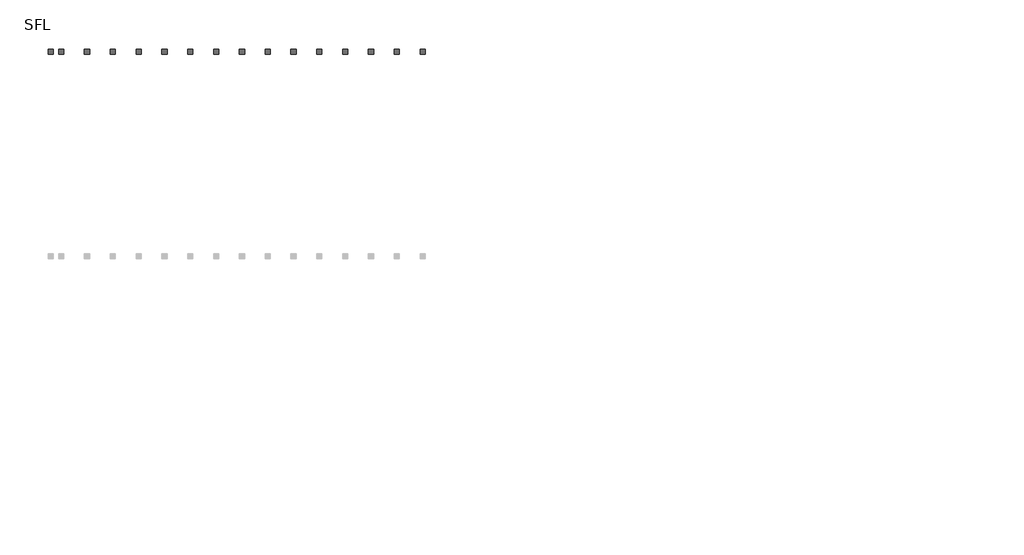
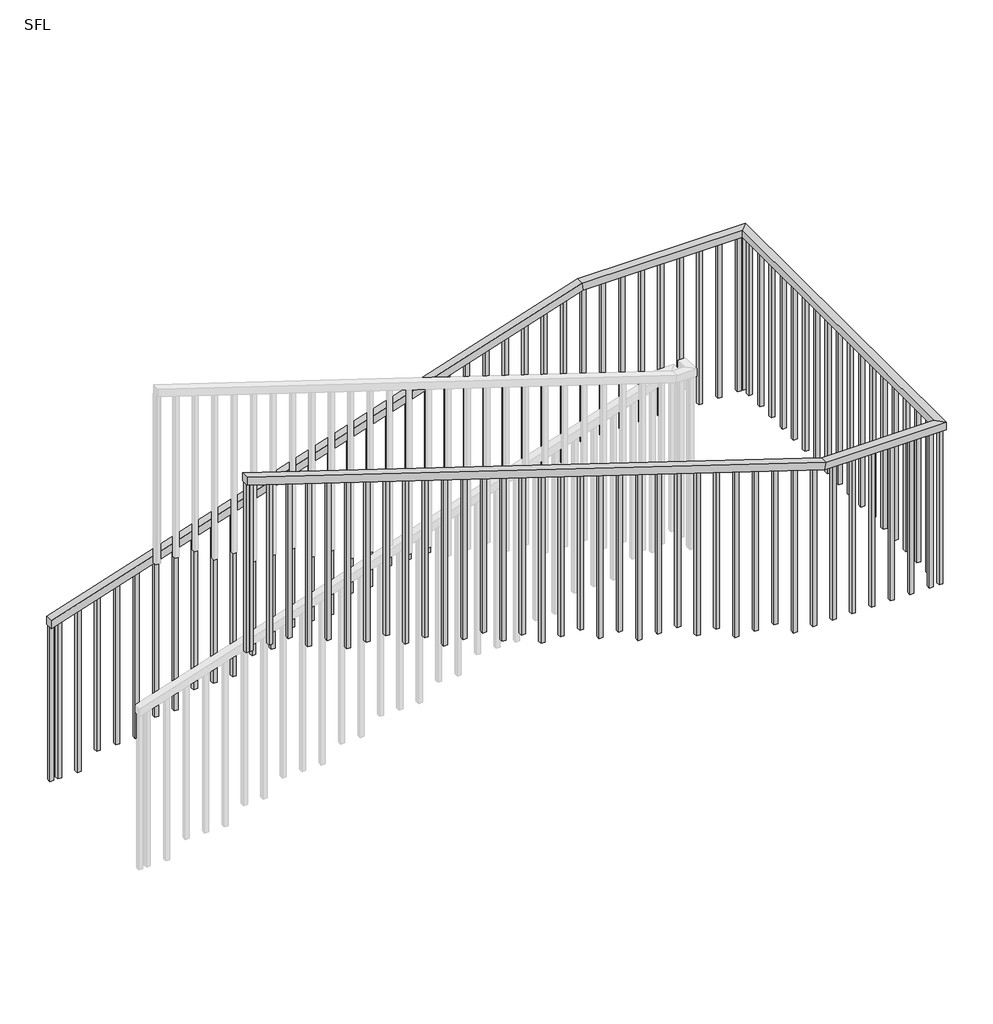
# One storey, part 2 of 2: 1 railing.
"""IFC4 building model written with IfcOpenShell, lengths in millimetres."""

from ifc_helpers import new_model, si_unit, frame, origin, place, context, project, spatial, polyline, outline, extrude, faceted_brep, element, save

model = new_model("IFC4")

# Units and contexts
model_context = context("Model", 3, world=origin())
ifc_project = project(units=[si_unit("LENGTHUNIT", "METRE", prefix="MILLI")], contexts=[model_context])

# Site, building, storey
site = spatial("IfcSite", under=ifc_project)
building = spatial("IfcBuilding", under=site)
storey = spatial("IfcBuildingStorey", under=building, Name="SFL", Elevation=6000.0)

# Railing
placement = place(None, origin())
element("IfcRailing", 1, ObjectType="1100mm", at=placement, inside=storey, context=model_context, shape_type="SolidModel", body=[
    faceted_brep([(-40149.9681829, 17835.7234223, 7799.9767904), (-40149.9681829, 17835.7234223, 7747.4487757), (-40149.9681829, 17785.7234223, 7747.4487757), (-40149.9681829, 17785.7234223, 7799.9767904), (-36733.6681829, 17835.7234223, 8899.9878906), (-36725.8169379, 17835.7234223, 8849.9878906), (-36725.8169379, 17785.7234223, 8849.9878906), (-36733.6681829, 17785.7234223, 8899.9878906), (-35651.74796, 17835.7234223, 8899.9878906), (-35651.74796, 17835.7234223, 8849.9878906), (-35701.74796, 17785.7234223, 8849.9878906), (-35701.74796, 17785.7234223, 8899.9878906), (-35651.74796, 15601.3234223, 8899.9878906), (-35651.74796, 15601.3234223, 8849.9878906), (-35701.74796, 15651.3234223, 8849.9878906), (-35701.74796, 15651.3234223, 8899.9878906), (-36423.0954556, 15601.3234223, 8899.9878906), (-36430.9467006, 15601.3234223, 8849.9878906), (-36430.9467006, 15651.3234223, 8849.9878906), (-36423.0954556, 15651.3234223, 8899.9878906), (-40149.9681829, 15601.3234223, 10100.0), (-40149.9681829, 15651.3234223, 10100.0), (-40149.9681829, 15651.3234223, 10047.4719853), (-40149.9681829, 15601.3234223, 10047.4719853)], [[[0, 1, 2, 3]], [[1, 0, 4, 5]], [[2, 1, 5, 6]], [[3, 2, 6, 7]], [[0, 3, 7, 4]], [[5, 4, 8, 9]], [[6, 5, 9, 10]], [[7, 6, 10, 11]], [[4, 7, 11, 8]], [[9, 8, 12, 13]], [[10, 9, 13, 14]], [[11, 10, 14, 15]], [[8, 11, 15, 12]], [[13, 12, 16, 17]], [[14, 13, 17, 18]], [[15, 14, 18, 19]], [[12, 15, 19, 16]], [[20, 21, 22, 23]], [[17, 16, 20, 23]], [[18, 17, 23, 22]], [[19, 18, 22, 21]], [[16, 19, 21, 20]]]),
    extrude(outline(polyline([(10031.9456028, -40101.74796), (10039.9953284, -40126.74796), (8899.9989909, -40126.74796), (8899.9989909, -40101.74796), (10031.9456028, -40101.74796)])), frame((0.0, 15613.8234223, 0.0), z_axis=(0.0, 1.0, 0.0), x_axis=(0.0, 0.0, 1.0)), (0.0, 0.0, 1.0), 25.0),
    extrude(outline(polyline([(9991.6969749, -39976.74796), (9999.7467005, -40001.74796), (8899.9989909, -40001.74796), (8899.9989909, -39976.74796), (9991.6969749, -39976.74796)])), frame((0.0, 15613.8234223, 0.0), z_axis=(0.0, 1.0, 0.0), x_axis=(0.0, 0.0, 1.0)), (0.0, 0.0, 1.0), 25.0),
    extrude(outline(polyline([(9951.448347, -39851.74796), (9959.4980726, -39876.74796), (8899.9989909, -39876.74796), (8899.9989909, -39851.74796), (9951.448347, -39851.74796)])), frame((0.0, 15613.8234223, 0.0), z_axis=(0.0, 1.0, 0.0), x_axis=(0.0, 0.0, 1.0)), (0.0, 0.0, 1.0), 25.0),
    extrude(outline(polyline([(9911.1997191, -39726.74796), (9919.2494447, -39751.74796), (8799.9979818, -39751.74796), (8799.9979818, -39726.74796), (9911.1997191, -39726.74796)])), frame((0.0, 15613.8234223, 0.0), z_axis=(0.0, 1.0, 0.0), x_axis=(0.0, 0.0, 1.0)), (0.0, 0.0, 1.0), 25.0),
    extrude(outline(polyline([(9870.9510912, -39601.74796), (9879.0008168, -39626.74796), (8799.9979818, -39626.74796), (8799.9979818, -39601.74796), (9870.9510912, -39601.74796)])), frame((0.0, 15613.8234223, 0.0), z_axis=(0.0, 1.0, 0.0), x_axis=(0.0, 0.0, 1.0)), (0.0, 0.0, 1.0), 25.0),
    extrude(outline(polyline([(9830.7024633, -39476.74796), (9838.7521889, -39501.74796), (8699.9969727, -39501.74796), (8699.9969727, -39476.74796), (9830.7024633, -39476.74796)])), frame((0.0, 15613.8234223, 0.0), z_axis=(0.0, 1.0, 0.0), x_axis=(0.0, 0.0, 1.0)), (0.0, 0.0, 1.0), 25.0),
    extrude(outline(polyline([(9790.4538354, -39351.74796), (9798.503561, -39376.74796), (8699.9969727, -39376.74796), (8699.9969727, -39351.74796), (9790.4538354, -39351.74796)])), frame((0.0, 15613.8234223, 0.0), z_axis=(0.0, 1.0, 0.0), x_axis=(0.0, 0.0, 1.0)), (0.0, 0.0, 1.0), 25.0),
    extrude(outline(polyline([(9750.2052075, -39226.74796), (9758.254933, -39251.74796), (8699.9969727, -39251.74796), (8699.9969727, -39226.74796), (9750.2052075, -39226.74796)])), frame((0.0, 15613.8234223, 0.0), z_axis=(0.0, 1.0, 0.0), x_axis=(0.0, 0.0, 1.0)), (0.0, 0.0, 1.0), 25.0),
    extrude(outline(polyline([(9710.0216346, -39101.74796), (9718.0713601, -39126.74796), (8599.9959635, -39126.74796), (8599.9959635, -39101.74796), (9710.0216346, -39101.74796)])), frame((0.0, 15613.8234223, 0.0), z_axis=(0.0, 1.0, 0.0), x_axis=(0.0, 0.0, 1.0)), (0.0, 0.0, 1.0), 25.0),
    extrude(outline(polyline([(9669.7730066, -38976.74796), (9677.8227322, -39001.74796), (8599.9959635, -39001.74796), (8599.9959635, -38976.74796), (9669.7730066, -38976.74796)])), frame((0.0, 15613.8234223, 0.0), z_axis=(0.0, 1.0, 0.0), x_axis=(0.0, 0.0, 1.0)), (0.0, 0.0, 1.0), 25.0),
    extrude(outline(polyline([(9629.5243787, -38851.74796), (9637.5741043, -38876.74796), (8499.9949544, -38876.74796), (8499.9949544, -38851.74796), (9629.5243787, -38851.74796)])), frame((0.0, 15613.8234223, 0.0), z_axis=(0.0, 1.0, 0.0), x_axis=(0.0, 0.0, 1.0)), (0.0, 0.0, 1.0), 25.0),
    extrude(outline(polyline([(9589.2757508, -38726.74796), (9597.3254764, -38751.74796), (8499.9949544, -38751.74796), (8499.9949544, -38726.74796), (9589.2757508, -38726.74796)])), frame((0.0, 15613.8234223, 0.0), z_axis=(0.0, 1.0, 0.0), x_axis=(0.0, 0.0, 1.0)), (0.0, 0.0, 1.0), 25.0),
    extrude(outline(polyline([(9549.0271229, -38601.74796), (9557.0768485, -38626.74796), (8499.9949544, -38626.74796), (8499.9949544, -38601.74796), (9549.0271229, -38601.74796)])), frame((0.0, 15613.8234223, 0.0), z_axis=(0.0, 1.0, 0.0), x_axis=(0.0, 0.0, 1.0)), (0.0, 0.0, 1.0), 25.0),
    extrude(outline(polyline([(9508.778495, -38476.74796), (9516.8282206, -38501.74796), (8399.9939453, -38501.74796), (8399.9939453, -38476.74796), (9508.778495, -38476.74796)])), frame((0.0, 15613.8234223, 0.0), z_axis=(0.0, 1.0, 0.0), x_axis=(0.0, 0.0, 1.0)), (0.0, 0.0, 1.0), 25.0),
    extrude(outline(polyline([(9468.5298671, -38351.74796), (9476.5795927, -38376.74796), (8399.9939453, -38376.74796), (8399.9939453, -38351.74796), (9468.5298671, -38351.74796)])), frame((0.0, 15613.8234223, 0.0), z_axis=(0.0, 1.0, 0.0), x_axis=(0.0, 0.0, 1.0)), (0.0, 0.0, 1.0), 25.0),
    extrude(outline(polyline([(9428.2812392, -38226.74796), (9436.3309648, -38251.74796), (8299.9929362, -38251.74796), (8299.9929362, -38226.74796), (9428.2812392, -38226.74796)])), frame((0.0, 15613.8234223, 0.0), z_axis=(0.0, 1.0, 0.0), x_axis=(0.0, 0.0, 1.0)), (0.0, 0.0, 1.0), 25.0),
    extrude(outline(polyline([(9388.0326113, -38101.74796), (9396.0823368, -38126.74796), (8299.9929362, -38126.74796), (8299.9929362, -38101.74796), (9388.0326113, -38101.74796)])), frame((0.0, 15613.8234223, 0.0), z_axis=(0.0, 1.0, 0.0), x_axis=(0.0, 0.0, 1.0)), (0.0, 0.0, 1.0), 25.0),
    extrude(outline(polyline([(9347.7839834, -37976.74796), (9355.8337089, -38001.74796), (8299.9929362, -38001.74796), (8299.9929362, -37976.74796), (9347.7839834, -37976.74796)])), frame((0.0, 15613.8234223, 0.0), z_axis=(0.0, 1.0, 0.0), x_axis=(0.0, 0.0, 1.0)), (0.0, 0.0, 1.0), 25.0),
    extrude(outline(polyline([(9307.5353554, -37851.74796), (9315.585081, -37876.74796), (8199.9919271, -37876.74796), (8199.9919271, -37851.74796), (9307.5353554, -37851.74796)])), frame((0.0, 15613.8234223, 0.0), z_axis=(0.0, 1.0, 0.0), x_axis=(0.0, 0.0, 1.0)), (0.0, 0.0, 1.0), 25.0),
    extrude(outline(polyline([(9267.2867275, -37726.74796), (9275.3364531, -37751.74796), (8199.9919271, -37751.74796), (8199.9919271, -37726.74796), (9267.2867275, -37726.74796)])), frame((0.0, 15613.8234223, 0.0), z_axis=(0.0, 1.0, 0.0), x_axis=(0.0, 0.0, 1.0)), (0.0, 0.0, 1.0), 25.0),
    extrude(outline(polyline([(9227.0380996, -37601.74796), (9235.0878252, -37626.74796), (8099.990918, -37626.74796), (8099.990918, -37601.74796), (9227.0380996, -37601.74796)])), frame((0.0, 15613.8234223, 0.0), z_axis=(0.0, 1.0, 0.0), x_axis=(0.0, 0.0, 1.0)), (0.0, 0.0, 1.0), 25.0),
    extrude(outline(polyline([(9186.7894717, -37476.74796), (9194.8391973, -37501.74796), (8099.990918, -37501.74796), (8099.990918, -37476.74796), (9186.7894717, -37476.74796)])), frame((0.0, 15613.8234223, 0.0), z_axis=(0.0, 1.0, 0.0), x_axis=(0.0, 0.0, 1.0)), (0.0, 0.0, 1.0), 25.0),
    extrude(outline(polyline([(9146.5408438, -37351.74796), (9154.5905694, -37376.74796), (8099.990918, -37376.74796), (8099.990918, -37351.74796), (9146.5408438, -37351.74796)])), frame((0.0, 15613.8234223, 0.0), z_axis=(0.0, 1.0, 0.0), x_axis=(0.0, 0.0, 1.0)), (0.0, 0.0, 1.0), 25.0),
    extrude(outline(polyline([(9106.2922159, -37226.74796), (9114.3419415, -37251.74796), (7999.9899089, -37251.74796), (7999.9899089, -37226.74796), (9106.2922159, -37226.74796)])), frame((0.0, 15613.8234223, 0.0), z_axis=(0.0, 1.0, 0.0), x_axis=(0.0, 0.0, 1.0)), (0.0, 0.0, 1.0), 25.0),
    extrude(outline(polyline([(9066.043588, -37101.74796), (9074.0933136, -37126.74796), (7999.9899089, -37126.74796), (7999.9899089, -37101.74796), (9066.043588, -37101.74796)])), frame((0.0, 15613.8234223, 0.0), z_axis=(0.0, 1.0, 0.0), x_axis=(0.0, 0.0, 1.0)), (0.0, 0.0, 1.0), 25.0),
    extrude(outline(polyline([(9025.7949601, -36976.74796), (9033.8446856, -37001.74796), (7899.9888997, -37001.74796), (7899.9888997, -36976.74796), (9025.7949601, -36976.74796)])), frame((0.0, 15613.8234223, 0.0), z_axis=(0.0, 1.0, 0.0), x_axis=(0.0, 0.0, 1.0)), (0.0, 0.0, 1.0), 25.0),
    extrude(outline(polyline([(8985.5463322, -36851.74796), (8993.5960577, -36876.74796), (7899.9888997, -36876.74796), (7899.9888997, -36851.74796), (8985.5463322, -36851.74796)])), frame((0.0, 15613.8234223, 0.0), z_axis=(0.0, 1.0, 0.0), x_axis=(0.0, 0.0, 1.0)), (0.0, 0.0, 1.0), 25.0),
    extrude(outline(polyline([(8945.2977042, -36726.74796), (8953.3474298, -36751.74796), (7899.9888997, -36751.74796), (7899.9888997, -36726.74796), (8945.2977042, -36726.74796)])), frame((0.0, 15613.8234223, 0.0), z_axis=(0.0, 1.0, 0.0), x_axis=(0.0, 0.0, 1.0)), (0.0, 0.0, 1.0), 25.0),
    extrude(outline(polyline([(8905.0490763, -36601.74796), (8913.0988019, -36626.74796), (7799.9878906, -36626.74796), (7799.9878906, -36601.74796), (8905.0490763, -36601.74796)])), frame((0.0, 15613.8234223, 0.0), z_axis=(0.0, 1.0, 0.0), x_axis=(0.0, 0.0, 1.0)), (0.0, 0.0, 1.0), 25.0),
    extrude(outline(polyline([(8864.8004484, -36476.74796), (8872.850174, -36501.74796), (7799.9878906, -36501.74796), (7799.9878906, -36476.74796), (8864.8004484, -36476.74796)])), frame((0.0, 15613.8234223, 0.0), z_axis=(0.0, 1.0, 0.0), x_axis=(0.0, 0.0, 1.0)), (0.0, 0.0, 1.0), 25.0),
    extrude(outline(polyline([(-36351.74796, 15613.8234223), (-36376.74796, 15613.8234223), (-36376.74796, 15638.8234223), (-36351.74796, 15638.8234223), (-36351.74796, 15613.8234223)])), frame((0.0, 0.0, 7799.9878906), z_axis=(0.0, 0.0, 1.0), x_axis=(1.0, 0.0, 0.0)), (0.0, 0.0, 1.0), 1050.0),
    extrude(outline(polyline([(-36226.74796, 15613.8234223), (-36251.74796, 15613.8234223), (-36251.74796, 15638.8234223), (-36226.74796, 15638.8234223), (-36226.74796, 15613.8234223)])), frame((0.0, 0.0, 7799.9878906), z_axis=(0.0, 0.0, 1.0), x_axis=(1.0, 0.0, 0.0)), (0.0, 0.0, 1.0), 1050.0),
    extrude(outline(polyline([(-36101.74796, 15613.8234223), (-36126.74796, 15613.8234223), (-36126.74796, 15638.8234223), (-36101.74796, 15638.8234223), (-36101.74796, 15613.8234223)])), frame((0.0, 0.0, 7799.9878906), z_axis=(0.0, 0.0, 1.0), x_axis=(1.0, 0.0, 0.0)), (0.0, 0.0, 1.0), 1050.0),
    extrude(outline(polyline([(-35976.74796, 15613.8234223), (-36001.74796, 15613.8234223), (-36001.74796, 15638.8234223), (-35976.74796, 15638.8234223), (-35976.74796, 15613.8234223)])), frame((0.0, 0.0, 7799.9878906), z_axis=(0.0, 0.0, 1.0), x_axis=(1.0, 0.0, 0.0)), (0.0, 0.0, 1.0), 1050.0),
    extrude(outline(polyline([(-35851.74796, 15613.8234223), (-35876.74796, 15613.8234223), (-35876.74796, 15638.8234223), (-35851.74796, 15638.8234223), (-35851.74796, 15613.8234223)])), frame((0.0, 0.0, 7799.9878906), z_axis=(0.0, 0.0, 1.0), x_axis=(1.0, 0.0, 0.0)), (0.0, 0.0, 1.0), 1050.0),
    extrude(outline(polyline([(-35726.74796, 15613.8234223), (-35751.74796, 15613.8234223), (-35751.74796, 15638.8234223), (-35726.74796, 15638.8234223), (-35726.74796, 15613.8234223)])), frame((0.0, 0.0, 7799.9878906), z_axis=(0.0, 0.0, 1.0), x_axis=(1.0, 0.0, 0.0)), (0.0, 0.0, 1.0), 1050.0),
    extrude(outline(polyline([(-35664.24796, 15760.7234223), (-35664.24796, 15735.7234223), (-35689.24796, 15735.7234223), (-35689.24796, 15760.7234223), (-35664.24796, 15760.7234223)])), frame((0.0, 0.0, 7799.9878906), z_axis=(0.0, 0.0, 1.0), x_axis=(1.0, 0.0, 0.0)), (0.0, 0.0, 1.0), 1050.0),
    extrude(outline(polyline([(-35664.24796, 15885.7234223), (-35664.24796, 15860.7234223), (-35689.24796, 15860.7234223), (-35689.24796, 15885.7234223), (-35664.24796, 15885.7234223)])), frame((0.0, 0.0, 7799.9878906), z_axis=(0.0, 0.0, 1.0), x_axis=(1.0, 0.0, 0.0)), (0.0, 0.0, 1.0), 1050.0),
    extrude(outline(polyline([(-35664.24796, 16010.7234223), (-35664.24796, 15985.7234223), (-35689.24796, 15985.7234223), (-35689.24796, 16010.7234223), (-35664.24796, 16010.7234223)])), frame((0.0, 0.0, 7799.9878906), z_axis=(0.0, 0.0, 1.0), x_axis=(1.0, 0.0, 0.0)), (0.0, 0.0, 1.0), 1050.0),
    extrude(outline(polyline([(-35664.24796, 16135.7234223), (-35664.24796, 16110.7234223), (-35689.24796, 16110.7234223), (-35689.24796, 16135.7234223), (-35664.24796, 16135.7234223)])), frame((0.0, 0.0, 7799.9878906), z_axis=(0.0, 0.0, 1.0), x_axis=(1.0, 0.0, 0.0)), (0.0, 0.0, 1.0), 1050.0),
    extrude(outline(polyline([(-35664.24796, 16260.7234223), (-35664.24796, 16235.7234223), (-35689.24796, 16235.7234223), (-35689.24796, 16260.7234223), (-35664.24796, 16260.7234223)])), frame((0.0, 0.0, 7799.9878906), z_axis=(0.0, 0.0, 1.0), x_axis=(1.0, 0.0, 0.0)), (0.0, 0.0, 1.0), 1050.0),
    extrude(outline(polyline([(-35664.24796, 16385.7234223), (-35664.24796, 16360.7234223), (-35689.24796, 16360.7234223), (-35689.24796, 16385.7234223), (-35664.24796, 16385.7234223)])), frame((0.0, 0.0, 7799.9878906), z_axis=(0.0, 0.0, 1.0), x_axis=(1.0, 0.0, 0.0)), (0.0, 0.0, 1.0), 1050.0),
    extrude(outline(polyline([(-35664.24796, 16510.7234223), (-35664.24796, 16485.7234223), (-35689.24796, 16485.7234223), (-35689.24796, 16510.7234223), (-35664.24796, 16510.7234223)])), frame((0.0, 0.0, 7799.9878906), z_axis=(0.0, 0.0, 1.0), x_axis=(1.0, 0.0, 0.0)), (0.0, 0.0, 1.0), 1050.0),
    extrude(outline(polyline([(-35664.24796, 16635.7234223), (-35664.24796, 16610.7234223), (-35689.24796, 16610.7234223), (-35689.24796, 16635.7234223), (-35664.24796, 16635.7234223)])), frame((0.0, 0.0, 7799.9878906), z_axis=(0.0, 0.0, 1.0), x_axis=(1.0, 0.0, 0.0)), (0.0, 0.0, 1.0), 1050.0),
    extrude(outline(polyline([(-35664.24796, 16760.7234223), (-35664.24796, 16735.7234223), (-35689.24796, 16735.7234223), (-35689.24796, 16760.7234223), (-35664.24796, 16760.7234223)])), frame((0.0, 0.0, 7799.9878906), z_axis=(0.0, 0.0, 1.0), x_axis=(1.0, 0.0, 0.0)), (0.0, 0.0, 1.0), 1050.0),
    extrude(outline(polyline([(-35664.24796, 16885.7234223), (-35664.24796, 16860.7234223), (-35689.24796, 16860.7234223), (-35689.24796, 16885.7234223), (-35664.24796, 16885.7234223)])), frame((0.0, 0.0, 7799.9878906), z_axis=(0.0, 0.0, 1.0), x_axis=(1.0, 0.0, 0.0)), (0.0, 0.0, 1.0), 1050.0),
    extrude(outline(polyline([(-35664.24796, 17010.7234223), (-35664.24796, 16985.7234223), (-35689.24796, 16985.7234223), (-35689.24796, 17010.7234223), (-35664.24796, 17010.7234223)])), frame((0.0, 0.0, 7799.9878906), z_axis=(0.0, 0.0, 1.0), x_axis=(1.0, 0.0, 0.0)), (0.0, 0.0, 1.0), 1050.0),
    extrude(outline(polyline([(-35664.24796, 17135.7234223), (-35664.24796, 17110.7234223), (-35689.24796, 17110.7234223), (-35689.24796, 17135.7234223), (-35664.24796, 17135.7234223)])), frame((0.0, 0.0, 7799.9878906), z_axis=(0.0, 0.0, 1.0), x_axis=(1.0, 0.0, 0.0)), (0.0, 0.0, 1.0), 1050.0),
    extrude(outline(polyline([(-35664.24796, 17260.7234223), (-35664.24796, 17235.7234223), (-35689.24796, 17235.7234223), (-35689.24796, 17260.7234223), (-35664.24796, 17260.7234223)])), frame((0.0, 0.0, 7799.9878906), z_axis=(0.0, 0.0, 1.0), x_axis=(1.0, 0.0, 0.0)), (0.0, 0.0, 1.0), 1050.0),
    extrude(outline(polyline([(-35664.24796, 17385.7234223), (-35664.24796, 17360.7234223), (-35689.24796, 17360.7234223), (-35689.24796, 17385.7234223), (-35664.24796, 17385.7234223)])), frame((0.0, 0.0, 7799.9878906), z_axis=(0.0, 0.0, 1.0), x_axis=(1.0, 0.0, 0.0)), (0.0, 0.0, 1.0), 1050.0),
    extrude(outline(polyline([(-35664.24796, 17510.7234223), (-35664.24796, 17485.7234223), (-35689.24796, 17485.7234223), (-35689.24796, 17510.7234223), (-35664.24796, 17510.7234223)])), frame((0.0, 0.0, 7799.9878906), z_axis=(0.0, 0.0, 1.0), x_axis=(1.0, 0.0, 0.0)), (0.0, 0.0, 1.0), 1050.0),
    extrude(outline(polyline([(-35664.24796, 17635.7234223), (-35664.24796, 17610.7234223), (-35689.24796, 17610.7234223), (-35689.24796, 17635.7234223), (-35664.24796, 17635.7234223)])), frame((0.0, 0.0, 7799.9878906), z_axis=(0.0, 0.0, 1.0), x_axis=(1.0, 0.0, 0.0)), (0.0, 0.0, 1.0), 1050.0),
    extrude(outline(polyline([(-35664.24796, 17760.7234223), (-35664.24796, 17735.7234223), (-35689.24796, 17735.7234223), (-35689.24796, 17760.7234223), (-35664.24796, 17760.7234223)])), frame((0.0, 0.0, 7799.9878906), z_axis=(0.0, 0.0, 1.0), x_axis=(1.0, 0.0, 0.0)), (0.0, 0.0, 1.0), 1050.0),
    extrude(outline(polyline([(-35724.9681829, 17823.2234223), (-35699.9681829, 17823.2234223), (-35699.9681829, 17798.2234223), (-35724.9681829, 17798.2234223), (-35724.9681829, 17823.2234223)])), frame((0.0, 0.0, 7799.9878906), z_axis=(0.0, 0.0, 1.0), x_axis=(1.0, 0.0, 0.0)), (0.0, 0.0, 1.0), 1050.0),
    extrude(outline(polyline([(-35849.9681829, 17823.2234223), (-35824.9681829, 17823.2234223), (-35824.9681829, 17798.2234223), (-35849.9681829, 17798.2234223), (-35849.9681829, 17823.2234223)])), frame((0.0, 0.0, 7799.9878906), z_axis=(0.0, 0.0, 1.0), x_axis=(1.0, 0.0, 0.0)), (0.0, 0.0, 1.0), 1050.0),
    extrude(outline(polyline([(-35974.9681829, 17823.2234223), (-35949.9681829, 17823.2234223), (-35949.9681829, 17798.2234223), (-35974.9681829, 17798.2234223), (-35974.9681829, 17823.2234223)])), frame((0.0, 0.0, 7799.9878906), z_axis=(0.0, 0.0, 1.0), x_axis=(1.0, 0.0, 0.0)), (0.0, 0.0, 1.0), 1050.0),
    extrude(outline(polyline([(-36099.9681829, 17823.2234223), (-36074.9681829, 17823.2234223), (-36074.9681829, 17798.2234223), (-36099.9681829, 17798.2234223), (-36099.9681829, 17823.2234223)])), frame((0.0, 0.0, 7799.9878906), z_axis=(0.0, 0.0, 1.0), x_axis=(1.0, 0.0, 0.0)), (0.0, 0.0, 1.0), 1050.0),
    extrude(outline(polyline([(-36224.9681829, 17823.2234223), (-36199.9681829, 17823.2234223), (-36199.9681829, 17798.2234223), (-36224.9681829, 17798.2234223), (-36224.9681829, 17823.2234223)])), frame((0.0, 0.0, 7799.9878906), z_axis=(0.0, 0.0, 1.0), x_axis=(1.0, 0.0, 0.0)), (0.0, 0.0, 1.0), 1050.0),
    extrude(outline(polyline([(-36349.9681829, 17823.2234223), (-36324.9681829, 17823.2234223), (-36324.9681829, 17798.2234223), (-36349.9681829, 17798.2234223), (-36349.9681829, 17823.2234223)])), frame((0.0, 0.0, 7799.9878906), z_axis=(0.0, 0.0, 1.0), x_axis=(1.0, 0.0, 0.0)), (0.0, 0.0, 1.0), 1050.0),
    extrude(outline(polyline([(-36474.9681829, 17823.2234223), (-36449.9681829, 17823.2234223), (-36449.9681829, 17798.2234223), (-36474.9681829, 17798.2234223), (-36474.9681829, 17823.2234223)])), frame((0.0, 0.0, 7799.9878906), z_axis=(0.0, 0.0, 1.0), x_axis=(1.0, 0.0, 0.0)), (0.0, 0.0, 1.0), 1050.0),
    extrude(outline(polyline([(-36599.9681829, 17823.2234223), (-36574.9681829, 17823.2234223), (-36574.9681829, 17798.2234223), (-36599.9681829, 17798.2234223), (-36599.9681829, 17823.2234223)])), frame((0.0, 0.0, 7799.9878906), z_axis=(0.0, 0.0, 1.0), x_axis=(1.0, 0.0, 0.0)), (0.0, 0.0, 1.0), 1050.0),
    extrude(outline(polyline([(-36724.9681829, 17823.2234223), (-36699.9681829, 17823.2234223), (-36699.9681829, 17798.2234223), (-36724.9681829, 17798.2234223), (-36724.9681829, 17823.2234223)])), frame((0.0, 0.0, 7799.9878906), z_axis=(0.0, 0.0, 1.0), x_axis=(1.0, 0.0, 0.0)), (0.0, 0.0, 1.0), 1050.0),
    extrude(outline(polyline([(7699.9868815, -36849.9681829), (7699.9868815, -36824.9681829), (8818.0622781, -36824.9681829), (8810.0125525, -36849.9681829), (7699.9868815, -36849.9681829)])), frame((0.0, 17798.2234223, 0.0), z_axis=(0.0, 1.0, 0.0), x_axis=(0.0, 0.0, 1.0)), (0.0, 0.0, 1.0), 25.0),
    extrude(outline(polyline([(7699.9868815, -36974.9681829), (7699.9868815, -36949.9681829), (8777.8136502, -36949.9681829), (8769.7639246, -36974.9681829), (7699.9868815, -36974.9681829)])), frame((0.0, 17798.2234223, 0.0), z_axis=(0.0, 1.0, 0.0), x_axis=(0.0, 0.0, 1.0)), (0.0, 0.0, 1.0), 25.0),
    extrude(outline(polyline([(7599.9858724, -37099.9681829), (7599.9858724, -37074.9681829), (8737.5650223, -37074.9681829), (8729.5152967, -37099.9681829), (7599.9858724, -37099.9681829)])), frame((0.0, 17798.2234223, 0.0), z_axis=(0.0, 1.0, 0.0), x_axis=(0.0, 0.0, 1.0)), (0.0, 0.0, 1.0), 25.0),
    extrude(outline(polyline([(7599.9858724, -37224.9681829), (7599.9858724, -37199.9681829), (8697.3163944, -37199.9681829), (8689.2666688, -37224.9681829), (7599.9858724, -37224.9681829)])), frame((0.0, 17798.2234223, 0.0), z_axis=(0.0, 1.0, 0.0), x_axis=(0.0, 0.0, 1.0)), (0.0, 0.0, 1.0), 25.0),
    extrude(outline(polyline([(7599.9858724, -37349.9681829), (7599.9858724, -37324.9681829), (8657.0677665, -37324.9681829), (8649.0180409, -37349.9681829), (7599.9858724, -37349.9681829)])), frame((0.0, 17798.2234223, 0.0), z_axis=(0.0, 1.0, 0.0), x_axis=(0.0, 0.0, 1.0)), (0.0, 0.0, 1.0), 25.0),
    extrude(outline(polyline([(7499.9848633, -37474.9681829), (7499.9848633, -37449.9681829), (8616.8191385, -37449.9681829), (8608.769413, -37474.9681829), (7499.9848633, -37474.9681829)])), frame((0.0, 17798.2234223, 0.0), z_axis=(0.0, 1.0, 0.0), x_axis=(0.0, 0.0, 1.0)), (0.0, 0.0, 1.0), 25.0),
    extrude(outline(polyline([(7499.9848633, -37599.9681829), (7499.9848633, -37574.9681829), (8576.5705106, -37574.9681829), (8568.5207851, -37599.9681829), (7499.9848633, -37599.9681829)])), frame((0.0, 17798.2234223, 0.0), z_axis=(0.0, 1.0, 0.0), x_axis=(0.0, 0.0, 1.0)), (0.0, 0.0, 1.0), 25.0),
    extrude(outline(polyline([(7399.9838542, -37724.9681829), (7399.9838542, -37699.9681829), (8536.3218827, -37699.9681829), (8528.2721571, -37724.9681829), (7399.9838542, -37724.9681829)])), frame((0.0, 17798.2234223, 0.0), z_axis=(0.0, 1.0, 0.0), x_axis=(0.0, 0.0, 1.0)), (0.0, 0.0, 1.0), 25.0),
    extrude(outline(polyline([(7399.9838542, -37849.9681829), (7399.9838542, -37824.9681829), (8496.0732548, -37824.9681829), (8488.0235292, -37849.9681829), (7399.9838542, -37849.9681829)])), frame((0.0, 17798.2234223, 0.0), z_axis=(0.0, 1.0, 0.0), x_axis=(0.0, 0.0, 1.0)), (0.0, 0.0, 1.0), 25.0),
    extrude(outline(polyline([(7399.9838542, -37974.9681829), (7399.9838542, -37949.9681829), (8455.8246269, -37949.9681829), (8447.7749013, -37974.9681829), (7399.9838542, -37974.9681829)])), frame((0.0, 17798.2234223, 0.0), z_axis=(0.0, 1.0, 0.0), x_axis=(0.0, 0.0, 1.0)), (0.0, 0.0, 1.0), 25.0),
    extrude(outline(polyline([(7299.9828451, -38099.9681829), (7299.9828451, -38074.9681829), (8415.575999, -38074.9681829), (8407.5262734, -38099.9681829), (7299.9828451, -38099.9681829)])), frame((0.0, 17798.2234223, 0.0), z_axis=(0.0, 1.0, 0.0), x_axis=(0.0, 0.0, 1.0)), (0.0, 0.0, 1.0), 25.0),
    extrude(outline(polyline([(7299.9828451, -38224.9681829), (7299.9828451, -38199.9681829), (8375.3273711, -38199.9681829), (8367.2776455, -38224.9681829), (7299.9828451, -38224.9681829)])), frame((0.0, 17798.2234223, 0.0), z_axis=(0.0, 1.0, 0.0), x_axis=(0.0, 0.0, 1.0)), (0.0, 0.0, 1.0), 25.0),
    extrude(outline(polyline([(7199.9818359, -38349.9681829), (7199.9818359, -38324.9681829), (8335.0787432, -38324.9681829), (8327.0290176, -38349.9681829), (7199.9818359, -38349.9681829)])), frame((0.0, 17798.2234223, 0.0), z_axis=(0.0, 1.0, 0.0), x_axis=(0.0, 0.0, 1.0)), (0.0, 0.0, 1.0), 25.0),
    extrude(outline(polyline([(7199.9818359, -38474.9681829), (7199.9818359, -38449.9681829), (8294.8301153, -38449.9681829), (8286.7803897, -38474.9681829), (7199.9818359, -38474.9681829)])), frame((0.0, 17798.2234223, 0.0), z_axis=(0.0, 1.0, 0.0), x_axis=(0.0, 0.0, 1.0)), (0.0, 0.0, 1.0), 25.0),
    extrude(outline(polyline([(7199.9818359, -38599.9681829), (7199.9818359, -38574.9681829), (8254.5814873, -38574.9681829), (8246.5317618, -38599.9681829), (7199.9818359, -38599.9681829)])), frame((0.0, 17798.2234223, 0.0), z_axis=(0.0, 1.0, 0.0), x_axis=(0.0, 0.0, 1.0)), (0.0, 0.0, 1.0), 25.0),
    extrude(outline(polyline([(7099.9808268, -38724.9681829), (7099.9808268, -38699.9681829), (8214.3328594, -38699.9681829), (8206.2831339, -38724.9681829), (7099.9808268, -38724.9681829)])), frame((0.0, 17798.2234223, 0.0), z_axis=(0.0, 1.0, 0.0), x_axis=(0.0, 0.0, 1.0)), (0.0, 0.0, 1.0), 25.0),
    extrude(outline(polyline([(7099.9808268, -38849.9681829), (7099.9808268, -38824.9681829), (8174.0842315, -38824.9681829), (8166.0345059, -38849.9681829), (7099.9808268, -38849.9681829)])), frame((0.0, 17798.2234223, 0.0), z_axis=(0.0, 1.0, 0.0), x_axis=(0.0, 0.0, 1.0)), (0.0, 0.0, 1.0), 25.0),
    extrude(outline(polyline([(6999.9798177, -38974.9681829), (6999.9798177, -38949.9681829), (8133.8356036, -38949.9681829), (8125.785878, -38974.9681829), (6999.9798177, -38974.9681829)])), frame((0.0, 17798.2234223, 0.0), z_axis=(0.0, 1.0, 0.0), x_axis=(0.0, 0.0, 1.0)), (0.0, 0.0, 1.0), 25.0),
    extrude(outline(polyline([(6999.9798177, -39099.9681829), (6999.9798177, -39074.9681829), (8093.5869757, -39074.9681829), (8085.5372501, -39099.9681829), (6999.9798177, -39099.9681829)])), frame((0.0, 17798.2234223, 0.0), z_axis=(0.0, 1.0, 0.0), x_axis=(0.0, 0.0, 1.0)), (0.0, 0.0, 1.0), 25.0),
    extrude(outline(polyline([(6999.9798177, -39224.9681829), (6999.9798177, -39199.9681829), (8053.3383478, -39199.9681829), (8045.2886222, -39224.9681829), (6999.9798177, -39224.9681829)])), frame((0.0, 17798.2234223, 0.0), z_axis=(0.0, 1.0, 0.0), x_axis=(0.0, 0.0, 1.0)), (0.0, 0.0, 1.0), 25.0),
    extrude(outline(polyline([(6899.9788086, -39349.9681829), (6899.9788086, -39324.9681829), (8013.0897199, -39324.9681829), (8005.0399943, -39349.9681829), (6899.9788086, -39349.9681829)])), frame((0.0, 17798.2234223, 0.0), z_axis=(0.0, 1.0, 0.0), x_axis=(0.0, 0.0, 1.0)), (0.0, 0.0, 1.0), 25.0),
    extrude(outline(polyline([(6899.9788086, -39474.9681829), (6899.9788086, -39449.9681829), (7972.841092, -39449.9681829), (7964.7913664, -39474.9681829), (6899.9788086, -39474.9681829)])), frame((0.0, 17798.2234223, 0.0), z_axis=(0.0, 1.0, 0.0), x_axis=(0.0, 0.0, 1.0)), (0.0, 0.0, 1.0), 25.0),
    extrude(outline(polyline([(6799.9777995, -39599.9681829), (6799.9777995, -39574.9681829), (7932.5924641, -39574.9681829), (7924.5427385, -39599.9681829), (6799.9777995, -39599.9681829)])), frame((0.0, 17798.2234223, 0.0), z_axis=(0.0, 1.0, 0.0), x_axis=(0.0, 0.0, 1.0)), (0.0, 0.0, 1.0), 25.0),
    extrude(outline(polyline([(6799.9777995, -39724.9681829), (6799.9777995, -39699.9681829), (7892.3438361, -39699.9681829), (7884.2941106, -39724.9681829), (6799.9777995, -39724.9681829)])), frame((0.0, 17798.2234223, 0.0), z_axis=(0.0, 1.0, 0.0), x_axis=(0.0, 0.0, 1.0)), (0.0, 0.0, 1.0), 25.0),
    extrude(outline(polyline([(6799.9777995, -39849.9681829), (6799.9777995, -39824.9681829), (7852.0952082, -39824.9681829), (7844.0454827, -39849.9681829), (6799.9777995, -39849.9681829)])), frame((0.0, 17798.2234223, 0.0), z_axis=(0.0, 1.0, 0.0), x_axis=(0.0, 0.0, 1.0)), (0.0, 0.0, 1.0), 25.0),
    extrude(outline(polyline([(6699.9767904, -39974.9681829), (6699.9767904, -39949.9681829), (7811.8465803, -39949.9681829), (7803.7968547, -39974.9681829), (6699.9767904, -39974.9681829)])), frame((0.0, 17798.2234223, 0.0), z_axis=(0.0, 1.0, 0.0), x_axis=(0.0, 0.0, 1.0)), (0.0, 0.0, 1.0), 25.0),
    extrude(outline(polyline([(6699.9767904, -40099.9681829), (6699.9767904, -40074.9681829), (7771.5979524, -40074.9681829), (7763.5482268, -40099.9681829), (6699.9767904, -40099.9681829)])), frame((0.0, 17798.2234223, 0.0), z_axis=(0.0, 1.0, 0.0), x_axis=(0.0, 0.0, 1.0)), (0.0, 0.0, 1.0), 25.0),
    extrude(outline(polyline([(-35664.24796, 15638.8234223), (-35664.24796, 15613.8234223), (-35689.24796, 15613.8234223), (-35689.24796, 15638.8234223), (-35664.24796, 15638.8234223)])), frame((0.0, 0.0, 7799.9878906), z_axis=(0.0, 0.0, 1.0), x_axis=(1.0, 0.0, 0.0)), (0.0, 0.0, 1.0), 1050.0),
    extrude(outline(polyline([(-35689.24796, 17823.2234223), (-35664.24796, 17823.2234223), (-35664.24796, 17798.2234223), (-35689.24796, 17798.2234223), (-35689.24796, 17823.2234223)])), frame((0.0, 0.0, 7799.9878906), z_axis=(0.0, 0.0, 1.0), x_axis=(1.0, 0.0, 0.0)), (0.0, 0.0, 1.0), 1050.0),
    extrude(outline(polyline([(10039.4222597, -40124.9681829), (10047.4719853, -40149.9681829), (8899.9989909, -40149.9681829), (8899.9989909, -40124.9681829), (10039.4222597, -40124.9681829)])), frame((0.0, 15613.8234223, 0.0), z_axis=(0.0, 1.0, 0.0), x_axis=(0.0, 0.0, 1.0)), (0.0, 0.0, 1.0), 25.0),
    extrude(outline(polyline([(6699.9767904, -40149.9681829), (6699.9767904, -40124.9681829), (7755.4985013, -40124.9681829), (7747.4487757, -40149.9681829), (6699.9767904, -40149.9681829)])), frame((0.0, 17798.2234223, 0.0), z_axis=(0.0, 1.0, 0.0), x_axis=(0.0, 0.0, 1.0)), (0.0, 0.0, 1.0), 25.0),
])

save(model, "model.ifc")

# Revit data of these elements
# Type "1100mm"
#   built-in parameter 1008612 = 0.019685 (stored number, unit not read)
#   built-in parameter 1008611 = 0.019685 (stored number, unit not read)
#   built-in parameter 1008609 = 0.902231 (stored number, unit not read)
#   built-in parameter 1008604 = 0.19685 (stored number, unit not read)
#   built-in parameter 1008603 = 0.164042 (stored number, unit not read)
#   Railing Height = 3' - 7.30709"
#   built-in parameter 1008630 = 2
#   built-in parameter 1008610 = 2
#   built-in parameter 1008608 = 1
#   built-in parameter 1008618 = Baluster_Square : 25mm
# Element 1 (IfcRailing, "1100mm")
#   Phase Created = New Construction
